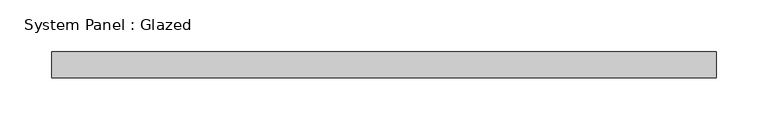
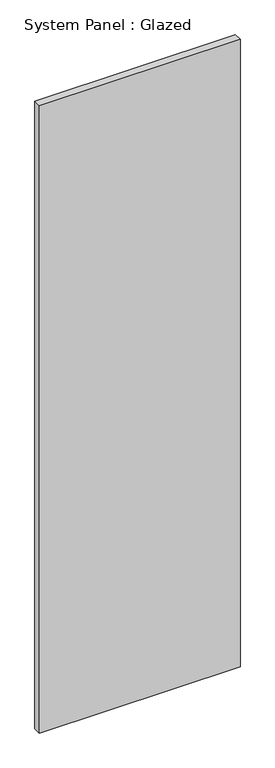
"""IFC4 building model written with IfcOpenShell, lengths in millimetres: plate geometry, System Panel : Glazed."""

from ifc_helpers import new_model, si_unit, origin, origin_with_axes, place, context, project, spatial, polyline, outline, extrude, source, transform, mapped, element, save


def system_panel_glazed_7e3d14c9(model_context):
    return source(origin(), model_context, "Body", "SweptSolid", [
        extrude(outline(polyline([(321.7333333, 19.05), (-321.7333333, 19.05), (-321.7333333, 44.45), (321.7333333, 44.45), (321.7333333, 19.05)])), origin_with_axes(), (0.0, 0.0, 1.0), 2127.25),
    ])


if __name__ == "__main__":
    model = new_model("IFC4")
    model_context = context("Model", 3, world=origin())
    ifc_project = project(units=[si_unit("LENGTHUNIT", "METRE", prefix="MILLI")], contexts=[model_context])
    site = spatial("IfcSite", under=ifc_project)
    building = spatial("IfcBuilding", under=site)
    placement = place(None, origin())
    system_panel_glazed_shape = system_panel_glazed_7e3d14c9(model_context)
    element("IfcPlate", 1, ObjectType="System Panel : Glazed", at=placement, inside=building, context=model_context, shape_type="MappedRepresentation", body=[
        mapped(system_panel_glazed_shape, transform((0.0, 0.0, 0.0), x_axis=(1.0, 0.0, 0.0), y_axis=(0.0, 1.0, 0.0), z_axis=(0.0, 0.0, 1.0))),
    ])
    save(model, "model.ifc")

# Revit data of these elements
# Type "System Panel : Glazed"
#   Construction Type Id = "GSP4R"
#   Analytic Construction = "1/8 in Pilkington single glazing"
#   Visual Light Transmittance = 0.9
#   Solar Heat Gain Coefficient = 0.86
#   Heat Transfer Coefficient (U) = 1.18115 BTU/(h·ft²·°F)
#   Define Thermal Properties by = 1
# Element 1 (IfcPlate, "System Panel : Glazed")
#   Materials on its faces: "Glass"
# Materials
#   "Glass": class "Glass", colour RGB 0 128 192, transparency 0.75, Description = "Soda Lime Glass", Cost = 0
